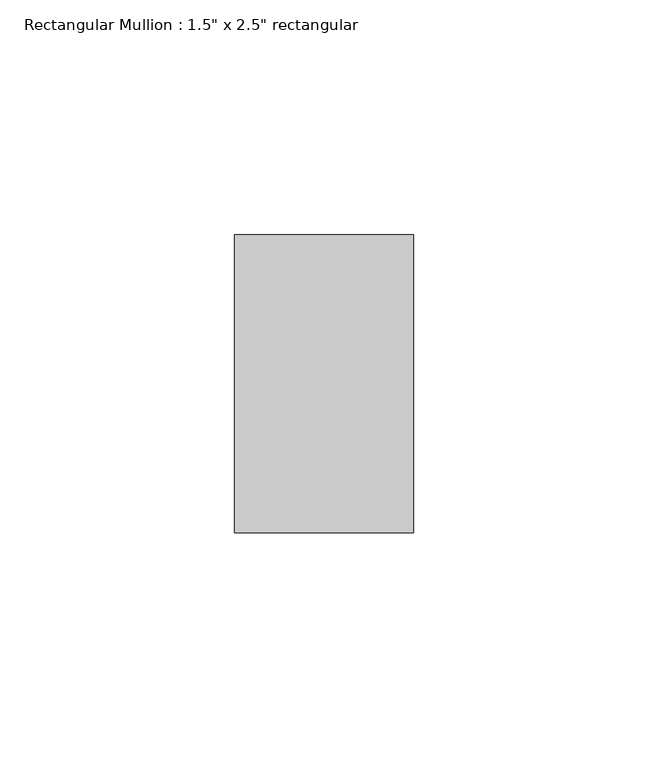
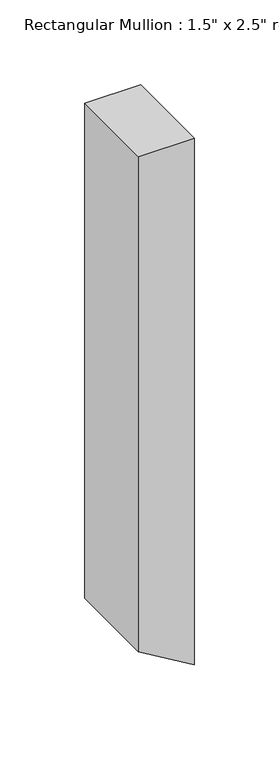
"""IFC4 building model written with IfcOpenShell, lengths in millimetres: member geometry."""

from ifc_helpers import new_model, si_unit, frame, origin, place, context, project, spatial, polyline, outline, extrude, source, transform, mapped, element, save


def member_354dc74f(model_context):
    return source(origin(), model_context, "Body", "SweptSolid", [
        extrude(outline(polyline([(0.0, 19.05), (0.0, -19.05), (-357.0487292, -19.05), (-379.6932431, 19.05), (0.0, 19.05)])), frame((0.0, -31.75, 0.0), z_axis=(0.0, 1.0, 0.0), x_axis=(0.0, 0.0, 1.0)), (0.0, 0.0, 1.0), 63.5),
    ])


if __name__ == "__main__":
    model = new_model("IFC4")
    model_context = context("Model", 3, world=origin())
    ifc_project = project(units=[si_unit("LENGTHUNIT", "METRE", prefix="MILLI")], contexts=[model_context])
    site = spatial("IfcSite", under=ifc_project)
    building = spatial("IfcBuilding", under=site)
    placement = place(None, origin())
    member_shape = member_354dc74f(model_context)
    element("IfcMember", 1, ObjectType="Rectangular Mullion : 1.5\" x 2.5\" rectangular", at=placement, inside=building, context=model_context, shape_type="MappedRepresentation", body=[
        mapped(member_shape, transform((0.0, 0.0, 0.0), x_axis=(1.0, 0.0, 0.0), y_axis=(0.0, 1.0, 0.0), z_axis=(0.0, 0.0, 1.0))),
    ])
    save(model, "model.ifc")

# Revit data of these elements
# Type "Rectangular Mullion : 1.5\" x 2.5\" rectangular"
#   built-in parameter 1007304 = 0.208333 (stored number, unit not read)
#   built-in parameter 1007301 = 0.0625 (stored number, unit not read)
#   built-in parameter 1007300 = 0.0625 (stored number, unit not read)
